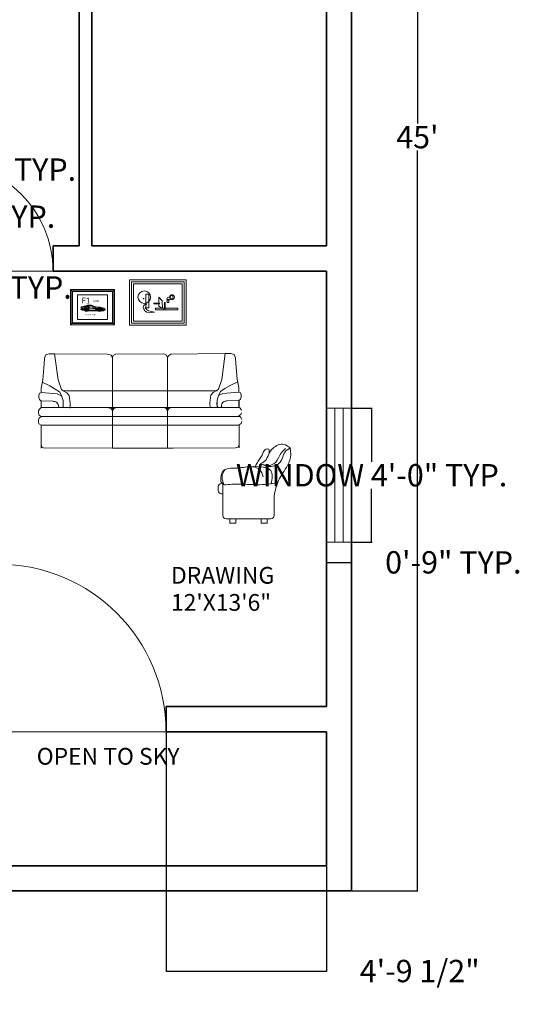
# Model space of a CAD drawing. Units: inches. Extents: x 125 to 976, y 231 to 853.
# Tile 15 of 16: x 736 to 915, y 231 to 584. Entities that reach past the tile are written whole.
import ezdxf

# ---------------------------------------------------------------- set-up
doc = ezdxf.new("R2010")
doc.units = ezdxf.units.IN
doc.header["$MEASUREMENT"] = 0
for name, color, linetype, lineweight in [('A-ANNO-DIMS', 2, 'Continuous', 18), ('A-AREA-IDEN', 7, 'Continuous', 18), ('A-DOOR', 3, 'Continuous', 18), ('A-FURN-ARTW', 9, 'Continuous', 13), ('A-GLAZ', 4, 'Continuous', 18), ('A-WALL', 7, 'Continuous', 35), ('Furniture', 8, 'Continuous', 15)]:
    doc.layers.add(name, color=color, linetype=linetype, lineweight=lineweight)
doc.styles.add('ITALICC', font='italicc', dxfattribs={"height": 240})
doc.styles.get("Standard").update_dxf_attribs({"font": 'italic8.shx'})
doc.dimstyles.get("Standard").update_dxf_attribs({"dimtxt": 8, "dimasz": 0.18, "dimexe": 0.18, "dimexo": 0.0625, "dimgap": 0.09, "dimtad": 0, "dimtih": 1, "dimtoh": 1, "dimdec": 4, "dimzin": 0, "dimdsep": 46, "dimlunit": 3, "dimtxsty": 'Standard', "dimcen": 0.09, "dimclrt": 4, "dimadec": 0, "dimazin": 0, "dimtfac": 1, "dimtdec": 4, "dimtofl": 0, "dimtmove": 0, "dimatfit": 3, "dimfxl": 1, "dimtolj": 1, "dimtzin": 0, "dimarcsym": 0})

# ---------------------------------------------------------------- blocks, each defined once
blk = doc.blocks.new('*D6')
at = {"layer": 'A-ANNO-DIMS', "color": 0, "lineweight": -2, "transparency": 16777216}
for p, q in [((855.26, 812.1), (878.96, 812.1)), ((878.78, 811.92), (878.78, 546.96)), ((878.78, 272.28), (878.78, 537.25)), ((846.26, 272.1), (878.96, 272.1))]:
    blk.add_line(p, q, dxfattribs=at)
at = {"layer": 'A-ANNO-DIMS', "color": 0, "transparency": 16777216}
for points in [[(878.75, 811.92), (878.81, 811.92), (878.78, 812.1)], [(878.75, 272.28), (878.81, 272.28), (878.78, 272.1)]]:
    blk.add_solid(points, dxfattribs=at)
at = {"layer": 'Defpoints', "color": 0, "transparency": 16777216}
for p in [(855.19, 812.1), (846.19, 272.1), (878.78, 272.1)]:
    blk.add_point(p, dxfattribs=at)
at = {"layer": 'A-ANNO-DIMS', "color": 0, "transparency": 16777216, "insert": (878.78, 542.1), "char_height": 8, "attachment_point": 5}
blk.add_mtext("\\A1;45'", dxfattribs=at)
blk = doc.blocks.new('SOFA-3SEAT')
for p, q in [((2, 30.21, -13.5), (2.15, 32.26, -13.5)), ((2.15, 32.26, -13.5), (2.61, 33.47, -13.5)), ((2.61, 33.47, -13.5), (3.76, 33.83, -13.5)), ((3.76, 33.83, -13.5), (5.77, 33.83, -13.5)), ((5.77, 33.83, -13.5), (24.71, 33.77, -13.5)), ((5.77, 33.83, -13.5), (7.07, 24.49, -13.5)), ((24.71, 33.77, -13.5), (26.18, 33.35, -13.5)), ((26.04, 33.37, -13.5), (26.5, 32.59, -13.5)), ((26.43, 32.53, -13.5), (26.87, 33.35, -13.5)), ((26.46, 32.58, -13.5), (26.52, 32.42, -13.5)), ((26.58, 32.81, -13.5), (26.58, 0, -13.5)), ((26.87, 33.35, -13.5), (27.73, 33.77, -13.5)), ((27.73, 33.77, -13.5), (44.96, 33.81, -13.5)), ((45.83, 33.4, -13.5), (44.96, 33.81, -13.5)), ((46.26, 32.57, -13.5), (45.83, 33.4, -13.5)), ((46.23, 32.63, -13.5), (46.18, 32.47, -13.5)), ((46.26, 32.63, -13.5), (46.69, 33.25, -13.5)), ((46.27, 0, -13.5), (46.27, 32.64, -13.5)), ((46.69, 33.25, -13.5), (47.38, 33.77, -13.5)), ((47.38, 33.77, -13.5), (66.92, 33.97, -13.5)), ((63.98, 33.86, -13.5), (63.98, 33.83, -13.5)), ((66.92, 33.97, -13.5), (65.66, 24.62, -13.5)), ((68.93, 33.98, -13.5), (66.92, 33.97, -13.5)), ((70.09, 33.62, -13.5), (68.93, 33.98, -13.5)), ((70.54, 32.42, -13.5), (70.09, 33.62, -13.5)), ((70.7, 30.37, -13.5), (70.54, 32.42, -13.5)), ((1.55, 24.55, -13.5), (2, 30.21, -13.5)), ((71.18, 24.71, -13.5), (70.7, 30.37, -13.5)), ((71.76, 21.75, -13.5), (71.18, 24.71, -13.5)), ((0.99, 21.59, -13.5), (1.55, 24.55, -13.5)), ((0.99, 21.59, -13.5), (0.99, 19.94, -13.5)), ((1.35, 23.64, -13.5), (4.11, 22.38, -13.5)), ((4.11, 22.38, -13.5), (5.97, 21.23, -13.5)), ((5.97, 21.23, -13.5), (7.53, 20.21, -13.5)), ((7.07, 24.49, -13.5), (8.28, 21.05, -13.5)), ((64.47, 21.18, -13.5), (63.92, 20.76, -13.5)), ((65.66, 24.62, -13.5), (64.47, 21.18, -13.5)), ((66.78, 21.37, -13.5), (65.23, 20.34, -13.5)), ((68.63, 22.53, -13.5), (66.78, 21.37, -13.5)), ((71.39, 23.81, -13.5), (68.63, 22.53, -13.5)), ((71.76, 21.75, -13.5), (71.76, 20.1, -13.5)), ((0.14, 18.15, -13.5), (0.18, 18.99, -13.5)), ((0.35, 17.44, -13.5), (0.14, 18.15, -13.5)), ((0.18, 18.99, -13.5), (0.38, 19.7, -13.5)), ((0.38, 19.7, -13.5), (0.98, 19.91, -13.5)), ((0.65, 19.79, -13.5), (0.65, 19.8, -13.5)), ((0.96, 19.94, -13.5), (6.7, 19.5, -13.5)), ((6.7, 19.5, -13.5), (8.26, 18.79, -13.5)), ((7.53, 20.21, -13.5), (8.33, 18.64, -13.5)), ((8.26, 18.79, -13.5), (8.83, 17.11, -13.5)), ((8.28, 21.05, -13.5), (8.83, 20.63, -13.5)), ((8.83, 20.63, -13.5), (63.95, 20.63, -13.5)), ((8.83, 20.63, -13.5), (10.14, 19.91, -13.5)), ((8.86, 20.63, -13.5), (8.86, 20.61, -13.5)), ((10.14, 19.91, -13.5), (10.98, 18.9, -13.5)), ((10.98, 18.9, -13.5), (11.34, 16.01, -13.5)), ((61.78, 19.02, -13.5), (61.43, 16.13, -13.5)), ((62.62, 20.03, -13.5), (61.78, 19.02, -13.5)), ((63.92, 20.76, -13.5), (62.62, 20.03, -13.5)), ((63.89, 20.76, -13.5), (63.89, 20.74, -13.5)), ((64.5, 18.92, -13.5), (63.94, 17.24, -13.5)), ((65.23, 20.34, -13.5), (64.43, 18.77, -13.5)), ((66.05, 19.64, -13.5), (64.5, 18.92, -13.5)), ((71.8, 20.1, -13.5), (66.05, 19.64, -13.5)), ((72.37, 19.87, -13.5), (71.78, 20.07, -13.5)), ((72.11, 19.95, -13.5), (72.11, 19.96, -13.5)), ((72.58, 19.16, -13.5), (72.37, 19.87, -13.5)), ((72.41, 17.61, -13.5), (72.62, 18.32, -13.5)), ((72.62, 18.32, -13.5), (72.58, 19.16, -13.5)), ((0.04, 13.5, -13.5), (0.49, 14.17, -13.5)), ((0.98, 16.94, -13.5), (0.35, 17.44, -13.5)), ((0.49, 14.17, -13.5), (1.01, 14.59, -13.5)), ((0.98, 16.95, -13.5), (5.28, 16.85, -13.5)), ((0.99, 16.95, -13.5), (0.99, 14.57, -13.5)), ((0.99, 14.57, -13.5), (0.99, 16.93, -13.5)), ((0.99, 14.57, -13.5), (71.86, 14.57, -13.5)), ((0.99, 14.57, -13.5), (0.99, 14.57, -13.5)), ((5.51, 16.75, -13.5), (5.27, 16.91, -13.5)), ((7.07, 14.84, -13.5), (7.3, 14.56, -13.5)), ((8.66, 14.72, -13.5), (8.26, 14.56, -13.5)), ((8.83, 14.88, -13.5), (8.66, 14.72, -13.5)), ((8.86, 15.75, -13.5), (8.81, 14.86, -13.5)), ((8.83, 17.11, -13.5), (8.86, 15.72, -13.5)), ((8.89, 14.57, -13.5), (8.89, 14.52, -13.5)), ((11.34, 16.01, -13.5), (11.34, 14.42, -13.5)), ((25.14, 14.53, -13.5), (26.09, 14.22, -13.5)), ((26.09, 14.22, -13.5), (26.52, 13.5, -13.5)), ((26.52, 13.5, -13.5), (27.04, 14.22, -13.5)), ((27.04, 14.22, -13.5), (27.73, 14.53, -13.5)), ((45.74, 14.26, -13.5), (45.05, 14.57, -13.5)), ((45.14, 14.53, -13.5), (46.17, 14.12, -13.5)), ((46.26, 13.54, -13.5), (45.74, 14.26, -13.5)), ((46.17, 14.12, -13.5), (46.26, 13.39, -13.5)), ((46.69, 14.27, -13.5), (46.26, 13.54, -13.5)), ((46.26, 13.39, -13.5), (46.6, 14.12, -13.5)), ((46.6, 14.12, -13.5), (47.29, 14.53, -13.5)), ((47.64, 14.58, -13.5), (46.69, 14.27, -13.5)), ((61.43, 16.13, -13.5), (61.44, 14.54, -13.5)), ((63.88, 14.69, -13.5), (63.88, 14.65, -13.5)), ((63.94, 17.24, -13.5), (63.91, 15.85, -13.5)), ((63.91, 15.87, -13.5), (63.97, 14.99, -13.5)), ((63.95, 15.01, -13.5), (64.12, 14.85, -13.5)), ((63.98, 17.37, -13.5), (63.98, 14.57, -13.5)), ((64.12, 14.85, -13.5), (64.51, 14.69, -13.5)), ((65.71, 14.98, -13.5), (65.48, 14.7, -13.5)), ((67.26, 16.9, -13.5), (67.49, 17.06, -13.5)), ((71.79, 17.11, -13.5), (67.48, 17, -13.5)), ((72.29, 14.34, -13.5), (71.76, 14.75, -13.5)), ((71.78, 17.11, -13.5), (71.79, 14.73, -13.5)), ((71.79, 14.73, -13.5), (71.78, 17.09, -13.5)), ((71.79, 17.1, -13.5), (72.41, 17.61, -13.5)), ((71.79, 14.73, -13.5), (71.79, 14.74, -13.5)), ((71.86, 17.15, -13.5), (71.86, 14.57, -13.5)), ((72.75, 13.67, -13.5), (72.29, 14.34, -13.5)), ((0.31, 10.84, -13.5), (0, 10.18, -13.5)), ((0.04, 12.58, -13.5), (0.04, 13.5, -13.5)), ((0.31, 11.91, -13.5), (0.04, 12.58, -13.5)), ((0.98, 11.41, -13.5), (0.31, 11.91, -13.5)), ((0.98, 11.45, -13.5), (0.31, 10.84, -13.5)), ((71.86, 11.42, -13.5), (0.99, 11.42, -13.5)), ((71.8, 11.42, -13.5), (71.8, 11.58, -13.5)), ((71.81, 11.57, -13.5), (72.48, 12.08, -13.5)), ((71.82, 11.61, -13.5), (72.49, 11, -13.5)), ((71.86, 11.6, -13.5), (71.86, 11.42, -13.5)), ((71.86, 11.6, -13.5), (71.86, 11.42, -13.5)), ((72.48, 12.08, -13.5), (72.75, 12.75, -13.5)), ((72.49, 11, -13.5), (72.8, 10.35, -13.5)), ((0, 10.18, -13.5), (0, 9.47, -13.5)), ((0, 9.47, -13.5), (0.19, 8.77, -13.5)), ((0.19, 8.77, -13.5), (0.98, 8.25, -13.5)), ((0.99, 8.27, -13.5), (71.86, 8.27, -13.5)), ((0.99, 0, -13.5), (0.99, 8.27, -13.5)), ((0.99, 8.27, -13.5), (0.99, 1.21, -13.5)), ((0.99, 8.27, -13.5), (0.99, 0, -13.5)), ((71.82, 8.43, -13.5), (71.81, 8.27, -13.5)), ((71.86, 0.16, -13.5), (71.82, 8.43, -13.5)), ((71.82, 8.43, -13.5), (71.85, 1.37, -13.5)), ((71.86, 0.16, -13.5), (71.82, 8.27, -13.5)), ((72.61, 8.93, -13.5), (71.83, 8.41, -13.5)), ((71.86, 8.43, -13.5), (71.86, 8.27, -13.5)), ((72.81, 9.64, -13.5), (72.61, 8.93, -13.5)), ((0.99, 1.21, -13.5), (1.35, 0.26, -13.5)), ((1.35, 0.26, -13.5), (2.3, 0, -13.5)), ((2.3, 0, -13.5), (70.55, 0.16, -13.5)), ((71.49, 0.42, -13.5), (70.55, 0.16, -13.5)), ((71.85, 1.37, -13.5), (71.49, 0.42, -13.5)), ((26.58, 0, -13.5), (46.27, 0, -13.5)), ((28.55, 0, -13.5), (48.23, 0, -13.5))]:
    blk.add_line(p, q)
for centre, start, end in [((5.4, 14.95, -13.5), 347.9294, 88.2763), ((67.38, 15.1, -13.5), 91.9867, 192.3335)]:
    blk.add_arc(centre, 1.85, start, end)
blk = doc.blocks.new('ART-FRAMED-ABSTRACT')
for p, q in [((0, 16.18), (20.24, 16.18)), ((0, 0), (0, 16.18)), ((0.71, 15.47), (19.53, 15.47)), ((0.71, 0.71), (0.71, 15.47)), ((0.71, 15.47), (19.53, 15.47)), ((0.71, 0.71), (0.71, 15.47)), ((1.42, 14.76), (18.82, 14.76)), ((1.42, 1.42), (1.42, 14.76)), ((18.82, 14.76), (18.82, 1.42)), ((19.53, 15.47), (19.53, 0.71)), ((19.53, 15.47), (19.53, 0.71)), ((20.24, 16.18), (20.24, 0)), ((5.79, 11.06), (6.88, 11.06)), ((5.79, 6.17), (5.79, 11.06)), ((6.88, 11.06), (6.88, 6.17)), ((6.88, 10.8), (6.95, 10.83)), ((6.88, 10.62), (6.95, 10.83)), ((3.12, 9.36), (3.17, 9.38)), ((3.14, 9.3), (3.17, 9.37)), ((4.91, 9.37), (5.13, 9.63)), ((4.91, 9.37), (5.18, 9.35)), ((5.18, 9.34), (5.13, 9.63)), ((5.66, 7.36), (5.76, 7.29)), ((5.76, 7.29), (5.79, 7.36)), ((5.79, 7.54), (5.85, 7.56)), ((5.81, 7.44), (5.85, 7.56)), ((8.71, 7.89), (10.73, 7.89)), ((8.71, 7.59), (8.71, 7.89)), ((10.73, 7.59), (8.71, 7.59)), ((10.55, 10.02), (11.64, 8.68)), ((10.55, 6.72), (10.55, 10.02)), ((10.73, 7.89), (10.73, 7.59)), ((11.64, 8.68), (11.75, 5.9)), ((12.76, 8.08), (12.51, 8.08)), ((12.51, 8.08), (12.51, 5.81)), ((12.76, 5.81), (12.76, 8.08)), ((13.43, 8.14), (13.43, 9.18)), ((13.43, 9.18), (14.11, 9.18)), ((14.11, 8.14), (13.43, 8.14)), ((14.11, 9.18), (14.11, 8.14)), ((5.53, 5.99), (5.8, 5.96)), ((5.54, 5.99), (5.75, 6.25)), ((5.81, 5.96), (5.75, 6.24)), ((6.88, 6.17), (5.79, 6.17)), ((17.28, 6.04), (9.28, 6.04)), ((9.28, 6.04), (9.28, 5.49)), ((9.28, 5.49), (17.28, 5.49)), ((11.75, 5.9), (10.55, 6.72)), ((12.04, 5.49), (12.21, 5.68)), ((12.24, 5.49), (12.21, 5.68)), ((12.51, 5.81), (12.76, 5.81)), ((17.28, 5.49), (17.28, 6.04)), ((20.24, 0), (0, 0)), ((19.53, 0.71), (0.71, 0.71)), ((19.53, 0.71), (0.71, 0.71)), ((18.82, 1.42), (1.42, 1.42))]:
    blk.add_line(p, q)
for centre, radius in [((5.29, 9.99), 2.26), ((15.21, 9.98), 0.893), ((13.98, 9.43), 0.565), ((15.09, 9.98), 0.578)]:
    blk.add_circle(centre, radius)
for points, knots in [([(6.1, 7.58), (5.6, 7.34), (4.53, 6.82), (5.68, 4.07), (7.64, 4.38), (8.96, 4.59)], [0, 0, 0, 0, 1.44737, 3.141992, 6.657621, 6.657621, 6.657621, 6.657621]), ([(6.1, 7.58), (5.92, 7.07), (5.29, 5.32), (7.43, 4.89), (8.96, 4.59)], [0, 0, 0, 0, 1.438871, 4.981716, 4.981716, 4.981716, 4.981716])]:
    blk.add_open_spline(points, degree=3, knots=knots)
blk = doc.blocks.new('WINDOW-48IN')
for p, q in [((0, 0), (0, 48)), ((0, 48), (9, 48)), ((3, 0), (3, 48)), ((6, 0), (6, 48)), ((9, 48), (9, 0)), ((9, 0), (0, 0))]:
    blk.add_line(p, q)
blk = doc.blocks.new('DOOR-39IN-RH')
for p, q in [((0, 39), (0, 0)), ((2, 38.95), (2, 0)), ((0, 0), (39, 0))]:
    blk.add_line(p, q)
blk.add_arc((0, 0), 39, 0, 90)
blk = doc.blocks.new('DOOR-60IN')
for p, q in [((0, 0), (0, 60)), ((2, 0), (2, 59.97)), ((60, 0), (0, 0))]:
    blk.add_line(p, q)
blk.add_arc((0, 0), 60, 0, 90)
blk = doc.blocks.new('*D24')
at = {"layer": 'A-ANNO-DIMS', "color": 0, "lineweight": -2, "transparency": 16777216}
for p, q in [((855.26, 444.98), (862.57, 444.98)), ((862.39, 444.8), (862.39, 425.84)), ((862.39, 397.16), (862.39, 416.13)), ((855.26, 396.98), (862.57, 396.98))]:
    blk.add_line(p, q, dxfattribs=at)
at = {"layer": 'A-ANNO-DIMS', "color": 0, "transparency": 16777216}
for points in [[(862.36, 444.8), (862.42, 444.8), (862.39, 444.98)], [(862.36, 397.16), (862.42, 397.16), (862.39, 396.98)]]:
    blk.add_solid(points, dxfattribs=at)
at = {"layer": 'Defpoints', "color": 0, "transparency": 16777216}
for p in [(855.19, 444.98), (862.39, 444.98), (855.19, 396.98)]:
    blk.add_point(p, dxfattribs=at)
at = {"layer": 'A-ANNO-DIMS', "color": 4, "transparency": 16777216, "insert": (862.39, 420.98), "char_height": 8, "attachment_point": 5}
blk.add_mtext('\\A1;WINDOW 4\'-0" TYP.', dxfattribs=at)
blk = doc.blocks.new('*D25')
at = {"layer": 'A-ANNO-DIMS', "color": 0, "lineweight": -2, "transparency": 16777216}
for p, q in [((846.19, 396.92), (846.19, 389.6)), ((855.19, 396.92), (855.19, 389.6)), ((846.37, 389.78), (855.01, 389.78)), ((855.19, 389.78), (855.37, 389.78))]:
    blk.add_line(p, q, dxfattribs=at)
at = {"layer": 'A-ANNO-DIMS', "color": 0, "transparency": 16777216}
for points in [[(846.37, 389.81), (846.37, 389.75), (846.19, 389.78)], [(855.01, 389.81), (855.01, 389.75), (855.19, 389.78)]]:
    blk.add_solid(points, dxfattribs=at)
at = {"layer": 'Defpoints', "color": 0, "transparency": 16777216}
for p in [(846.19, 396.98), (855.19, 396.98), (855.19, 389.78)]:
    blk.add_point(p, dxfattribs=at)
at = {"layer": 'A-ANNO-DIMS', "color": 4, "transparency": 16777216, "insert": (891.65, 389.78), "char_height": 8, "attachment_point": 5}
blk.add_mtext('\\A1;0\'-9" TYP.', dxfattribs=at)
blk = doc.blocks.new('*D38')
at = {"layer": 'A-ANNO-DIMS', "color": 0, "lineweight": -2, "transparency": 16777216}
for p, q in [((694.22, 533.1), (700.18, 533.1)), ((700, 532.92), (700, 518.46)), ((700, 494.28), (700, 508.75)), ((694.22, 494.1), (700.18, 494.1))]:
    blk.add_line(p, q, dxfattribs=at)
at = {"layer": 'A-ANNO-DIMS', "color": 0, "transparency": 16777216}
for points in [[(699.97, 532.92), (700.03, 532.92), (700, 533.1)], [(699.97, 494.28), (700.03, 494.28), (700, 494.1)]]:
    blk.add_solid(points, dxfattribs=at)
at = {"layer": 'Defpoints', "color": 0, "transparency": 16777216}
for p in [(694.15, 533.1), (700, 533.1), (694.15, 494.1)]:
    blk.add_point(p, dxfattribs=at)
at = {"layer": 'A-ANNO-DIMS', "color": 4, "transparency": 16777216, "insert": (700, 513.6), "char_height": 8, "attachment_point": 5}
blk.add_mtext('\\A1;LH DOOR 3\'-3" TYP.', dxfattribs=at)
blk = doc.blocks.new('*D39')
at = {"layer": 'A-ANNO-DIMS', "color": 0, "lineweight": -2, "transparency": 16777216}
for p, q in [((655.15, 494.04), (655.15, 488.07)), ((694.15, 494.04), (694.15, 488.07)), ((655.33, 488.25), (693.97, 488.25)), ((694.15, 488.25), (694.33, 488.25))]:
    blk.add_line(p, q, dxfattribs=at)
at = {"layer": 'A-ANNO-DIMS', "color": 0, "transparency": 16777216}
for points in [[(655.33, 488.28), (655.33, 488.22), (655.15, 488.25)], [(693.97, 488.28), (693.97, 488.22), (694.15, 488.25)]]:
    blk.add_solid(points, dxfattribs=at)
at = {"layer": 'Defpoints', "color": 0, "transparency": 16777216}
for p in [(655.15, 494.1), (694.15, 494.1), (694.15, 488.25)]:
    blk.add_point(p, dxfattribs=at)
at = {"layer": 'A-ANNO-DIMS', "color": 4, "transparency": 16777216, "insert": (730.61, 488.25), "char_height": 8, "attachment_point": 5}
blk.add_mtext('\\A1;3\'-3" TYP.', dxfattribs=at)
blk = doc.blocks.new('*D48')
at = {"layer": 'A-ANNO-DIMS', "color": 0, "lineweight": -2, "transparency": 16777216}
for p, q in [((609.57, 526.38), (609.57, 530.63)), ((609.75, 530.45), (636.95, 530.45)), ((637.13, 526.38), (637.13, 530.63)), ((637.13, 530.45), (637.31, 530.45))]:
    blk.add_line(p, q, dxfattribs=at)
at = {"layer": 'A-ANNO-DIMS', "color": 0, "transparency": 16777216}
for points in [[(609.75, 530.48), (609.75, 530.42), (609.57, 530.45)], [(636.95, 530.48), (636.95, 530.42), (637.13, 530.45)]]:
    blk.add_solid(points, dxfattribs=at)
at = {"layer": 'Defpoints', "color": 0, "transparency": 16777216}
for p in [(637.13, 530.45), (609.57, 526.32), (637.13, 526.32)]:
    blk.add_point(p, dxfattribs=at)
at = {"layer": 'A-ANNO-DIMS', "color": 4, "transparency": 16777216, "insert": (709.21, 530.45), "char_height": 8, "attachment_point": 5}
blk.add_mtext('\\A1;SINK 2\'-3 1/2" TYP.', dxfattribs=at)
blk = doc.blocks.new('*D61')
at = {"layer": 'A-ANNO-DIMS', "color": 0, "lineweight": -2, "transparency": 16777216}
for p, q in [((788.78, 329.04), (788.78, 243.22)), ((846.19, 329.04), (846.19, 243.22)), ((788.96, 243.4), (846.01, 243.4)), ((846.19, 243.4), (846.37, 243.4))]:
    blk.add_line(p, q, dxfattribs=at)
at = {"layer": 'A-ANNO-DIMS', "color": 0, "transparency": 16777216}
for points in [[(788.96, 243.43), (788.96, 243.37), (788.78, 243.4)], [(846.01, 243.43), (846.01, 243.37), (846.19, 243.4)]]:
    blk.add_solid(points, dxfattribs=at)
at = {"layer": 'Defpoints', "color": 0, "transparency": 16777216}
for p in [(788.78, 329.1), (846.19, 329.1), (846.19, 243.4)]:
    blk.add_point(p, dxfattribs=at)
at = {"layer": 'A-ANNO-DIMS', "color": 4, "transparency": 16777216, "insert": (879.61, 243.4), "char_height": 8, "attachment_point": 5}
blk.add_mtext('\\A1;4\'-9 1/2"', dxfattribs=at)

msp = doc.modelspace()

# ---------------------------------------------------------------- linework, layer by layer
at = {"layer": 'A-FURN-ARTW'}
for p, q in [((754.60231, 487.494), (770.35031, 487.494)), ((754.60231, 487.494), (754.60231, 474.8956)), ((755.29522, 486.80109), (754.60231, 487.494)), ((755.07475, 487.02156), (769.87787, 487.02156)), ((755.07475, 487.02156), (755.07475, 475.36804)), ((755.23223, 486.86408), (769.72039, 486.86408)), ((755.23223, 486.86408), (755.23223, 475.52552)), ((755.29522, 486.80109), (769.6574, 486.80109)), ((755.29522, 486.80109), (755.29522, 475.58851)), ((769.6574, 486.80109), (770.35031, 487.494)), ((769.6574, 486.80109), (769.6574, 475.58851)), ((769.72039, 486.86408), (769.72039, 475.52552)), ((769.87787, 487.02156), (769.87787, 475.36804)), ((770.35031, 487.494), (770.35031, 474.8956)), ((757.12199, 485.60424), (767.83063, 485.60424)), ((757.12199, 485.60424), (757.12199, 476.78536)), ((767.83063, 485.60424), (767.83063, 476.78536)), ((758.28026, 480.5186), (758.34094, 480.76133)), ((758.31237, 480.5105), (758.28291, 480.5105)), ((758.3117, 480.42103), (758.28293, 480.4868)), ((758.33795, 480.50224), (758.31237, 480.5105)), ((758.33128, 480.50425), (759.47693, 480.30077)), ((758.33229, 480.52296), (758.39189, 480.76133)), ((758.38079, 480.38642), (758.33496, 480.49117)), ((758.36266, 481.31769), (758.41208, 480.89761)), ((758.38737, 480.83583), (758.41208, 480.89761)), ((758.39972, 480.81112), (758.38737, 480.83583)), ((758.38737, 480.78641), (758.39972, 480.81112)), ((758.38889, 480.83583), (759.73849, 480.83583)), ((758.38889, 480.79877), (759.73214, 480.79877)), ((758.41544, 481.29201), (758.46263, 480.89091)), ((758.4406, 480.83583), (758.46263, 480.89091)), ((758.45824, 480.30563), (759.47462, 480.12512)), ((758.71184, 480.14222), (758.57964, 480.20951)), ((758.7086, 480.83583), (758.65918, 481.30533)), ((758.75802, 480.74935), (758.75802, 480.65051)), ((758.75802, 480.74935), (759.09161, 480.74935)), ((758.75802, 480.65051), (759.09161, 480.65051)), ((758.77379, 481.30451), (759.74709, 481.35476)), ((758.83434, 480.20886), (758.8198, 480.24279)), ((758.9079, 480.15048), (759.62949, 480.02232)), ((759.09161, 480.74935), (759.09161, 480.65051)), ((759.15339, 481.37946), (759.74644, 481.37946)), ((759.47462, 480.24279), (759.47462, 480.12512)), ((760.68637, 481.36279), (760.62387, 481.83335)), ((760.71087, 481.36605), (760.64837, 481.8366)), ((760.66826, 480.83615), (764.36543, 480.6804)), ((760.67502, 480.79877), (764.37001, 480.6431)), ((760.75956, 479.88449), (761.03138, 479.88449)), ((761.0808, 479.93391), (760.77192, 479.9092)), ((762.28859, 481.82292), (760.92169, 481.79935)), ((761.05609, 481.3424), (760.92169, 481.79935)), ((760.95361, 479.97939), (760.93253, 480.24279)), ((762.00687, 481.79335), (760.95455, 481.7752)), ((761.07979, 481.34937), (760.95455, 481.7752)), ((760.95725, 480.13159), (764.24854, 480.13159)), ((760.95725, 479.98333), (764.21901, 479.98333)), ((761.00287, 479.93391), (764.21901, 479.93391)), ((761.03138, 479.88449), (761.09315, 479.9092)), ((761.72327, 481.26827), (761.05609, 481.3424)), ((761.0808, 481.13236), (761.37732, 481.13236)), ((761.0808, 481.04587), (761.0808, 481.13236)), ((761.37732, 481.08294), (761.0808, 481.08294)), ((761.37732, 481.04587), (761.0808, 481.04587)), ((761.09315, 479.9092), (761.34026, 479.9092)), ((761.34026, 479.9092), (761.35261, 479.87213)), ((761.35261, 479.87213), (761.82211, 479.87213)), ((761.37732, 481.13236), (761.37732, 481.04587)), ((761.82211, 479.87213), (761.92095, 479.88449)), ((761.92095, 479.88449), (762.01979, 479.89684)), ((761.96424, 481.81733), (763.01468, 481.22646)), ((762.01314, 481.81817), (763.06137, 481.22854)), ((762.01979, 479.89684), (762.09392, 479.89684)), ((762.09392, 479.89684), (762.11863, 479.87213)), ((762.11095, 481.81986), (763.15355, 481.23339)), ((762.11863, 479.87213), (762.20512, 479.87213)), ((762.20512, 479.87213), (762.2916, 479.88449)), ((762.28859, 481.82292), (763.50241, 481.26065)), ((762.2916, 479.88449), (762.45222, 479.88449)), ((762.45222, 479.88449), (762.46458, 479.87213)), ((762.46458, 479.87213), (762.56342, 479.87213)), ((762.5669, 481.39311), (762.52131, 481.22594)), ((762.56342, 479.87213), (762.60048, 479.88449)), ((762.63842, 481.37361), (762.59625, 481.21898)), ((762.60048, 479.88449), (763.28002, 479.88449)), ((762.66226, 481.36711), (762.62519, 481.2312)), ((762.62519, 481.2312), (762.6499, 481.20649)), ((762.62519, 481.2312), (762.94643, 481.2312)), ((762.6499, 481.20649), (762.92172, 481.21885)), ((762.67461, 481.39182), (762.66226, 481.36711)), ((762.95878, 481.2312), (762.66226, 481.35475)), ((762.95878, 481.2312), (762.67461, 481.39182)), ((762.71168, 481.18178), (762.71168, 481.21885)), ((762.85994, 481.18178), (762.71168, 481.18178)), ((762.85994, 481.21885), (762.85994, 481.18178)), ((764.68851, 481.19413), (762.85994, 481.19413)), ((762.92172, 481.21885), (762.95878, 481.2312)), ((763.28002, 479.88449), (763.30473, 479.87213)), ((763.30473, 479.87213), (763.40357, 479.87213)), ((763.40357, 479.87213), (763.41593, 479.88449)), ((763.41593, 479.88449), (763.78658, 479.89684)), ((763.57173, 481.26606), (764.47103, 481.19413)), ((763.73716, 480.20572), (763.62596, 480.20572)), ((763.76187, 480.58873), (763.63832, 480.58873)), ((763.70377, 481.3041), (763.6908, 481.25518)), ((763.73558, 481.30145), (763.70377, 481.3041)), ((763.74492, 481.28939), (763.73558, 481.30145)), ((763.76187, 480.58873), (763.73716, 480.20572)), ((763.74492, 481.28939), (764.68851, 481.19413)), ((763.78658, 479.89684), (764.1943, 479.89684)), ((763.98426, 480.20572), (763.87307, 480.20572)), ((764.00897, 480.57638), (763.88542, 480.57638)), ((764.00897, 480.57638), (763.98426, 480.20572)), ((764.1943, 479.89684), (764.26843, 479.89684)), ((764.24854, 480.13159), (764.21901, 479.98333)), ((764.21901, 479.98333), (764.21901, 479.93391)), ((764.26843, 479.89684), (764.29314, 479.92155)), ((764.29314, 479.92155), (764.36727, 479.9092)), ((764.36727, 479.9092), (764.41669, 479.9092)), ((764.41669, 479.9092), (764.43723, 479.91946)), ((765.57808, 479.92155), (765.52906, 479.91338)), ((765.65221, 479.94626), (765.57808, 479.92155)), ((765.75105, 479.9092), (765.65221, 479.94626)), ((765.70762, 480.58675), (766.67803, 480.54587)), ((765.71532, 480.62353), (766.66898, 480.58335)), ((765.81283, 479.9092), (765.75105, 479.9092)), ((765.81283, 480.03275), (765.79911, 480.26415)), ((765.81283, 480.03275), (765.81283, 479.85978)), ((765.87531, 480.53022), (766.20417, 480.51637)), ((765.87531, 480.53022), (765.9003, 480.43024)), ((765.9003, 480.43024), (766.24186, 480.41585)), ((766.20417, 480.51637), (766.24186, 480.41585)), ((766.3018, 479.89084), (766.40588, 479.98333)), ((766.40588, 479.98333), (766.61592, 480.05746)), ((766.61592, 480.05746), (766.66534, 480.10688)), ((766.66898, 480.58335), (766.75364, 480.2326)), ((766.67803, 480.54587), (766.88975, 480.56691)), ((766.70701, 480.586), (766.84673, 480.59988)), ((766.7307, 480.48561), (766.77734, 480.2924)), ((766.75228, 480.516), (766.89341, 480.53002)), ((766.76418, 480.16866), (766.80124, 480.19337)), ((766.76677, 480.33617), (766.92479, 480.30456)), ((766.87537, 480.30456), (766.77678, 480.2947)), ((766.78365, 480.26623), (766.80124, 480.19337)), ((766.7897, 480.19625), (766.90008, 480.16866)), ((766.94951, 480.30456), (766.87537, 480.30456)), ((766.89341, 480.53002), (766.94951, 480.30456)), ((766.91471, 480.54296), (766.98479, 480.27431)), ((757.12199, 476.78536), (767.83063, 476.78536)), ((755.29522, 475.58851), (754.60231, 474.8956)), ((754.60231, 474.8956), (770.35031, 474.8956)), ((755.07475, 475.36804), (769.87787, 475.36804)), ((755.23223, 475.52552), (769.72039, 475.52552)), ((755.29522, 475.58851), (769.6574, 475.58851)), ((769.6574, 475.58851), (770.35031, 474.8956))]:
    msp.add_line(p, q, dxfattribs=at)
for centre, radius in [((760.22829, 480.25514), 0.64247), ((760.22829, 480.25514), 0.49421), ((760.22829, 480.25514), 0.44479), ((760.22829, 480.25514), 0.2471), ((760.22829, 480.25514), 0.19768), ((760.08003, 480.25514), 0.02471), ((760.22829, 480.25514), 0.07413), ((760.18247, 480.39615), 0.02471), ((760.18247, 480.11414), 0.02471), ((760.34824, 480.34229), 0.02471), ((760.34824, 480.168), 0.02471), ((764.98503, 480.25514), 0.64247), ((764.98503, 480.25514), 0.49421), ((764.98503, 480.25514), 0.44479), ((764.98503, 480.25514), 0.2471), ((764.98503, 480.25514), 0.19768), ((764.83677, 480.25514), 0.02471), ((764.98503, 480.25514), 0.07413), ((764.93922, 480.39615), 0.02471), ((764.93922, 480.11414), 0.02471), ((765.10498, 480.34229), 0.02471), ((765.10498, 480.168), 0.02471)]:
    msp.add_circle(centre, radius, dxfattribs=at)
for centre, radius, start, end in [((758.32821, 480.50661), 0.04942, 165.9637565, 203.6293777), ((758.49281, 480.50027), 0.19768, 203.6293777, 259.9289375), ((758.38024, 480.51098), 0.04942, 165.9637565, 203.6293777), ((758.38889, 480.74935), 0.04942, 90, 165.9637565), ((758.45963, 485.16796), 3.85149, 268.5572, 280.3771181), ((758.37356, 481.26891), 0.04783, 28.8809621, 100.3164566), ((757.77157, 481.03149), 0.64307, 353.8619855, 19.3390879), ((758.51662, 480.44585), 0.14826, 203.6293777, 259.9289375), ((758.43983, 480.74935), 0.04942, 90, 165.9637565), ((757.78767, 481.03149), 0.64307, 353.8619855, 19.3390879), ((758.88575, 481.1779), 0.4815, 179.5142446, 197.7013491), ((758.45963, 485.16796), 3.8762, 269.3467381, 274.6487218), ((758.85814, 480.10092), 0.29891, 143.8021327, 158.6989451), ((758.82923, 480.12635), 0.11845, 100.5968558, 172.3030214), ((758.92519, 480.2478), 0.09884, 203.1985905, 259.9289375), ((763.44988, 470.16664), 12.00779, 103.37068, 110.9656649), ((760.20358, 480.24279), 0.72896, 0, 180), ((760.20358, 480.48989), 0.6054, 34.8499046, 145.1500954), ((760.20358, 480.24279), 0.75367, 51.9345418, 128.1046218), ((760.0615, 469.35582), 12.02777, 85.2567236, 91.5009845), ((760.0615, 469.35582), 12.00306, 84.4178875, 91.5009845), ((760.22829, 480.25514), 0.42008, 155.4545455, 178.5415782), ((760.22829, 480.25514), 0.42008, 188.1818182, 211.268851), ((760.22829, 480.25514), 0.39537, 159.1289708, 182.4346937), ((760.22829, 480.25514), 0.39537, 191.8562435, 215.1619665), ((760.22829, 480.25514), 0.37066, 161.8383609, 185.4083365), ((760.22829, 480.25514), 0.37066, 194.5656336, 218.1356092), ((760.22829, 480.25514), 0.42008, 122.7272727, 145.8143055), ((760.22829, 480.25514), 0.39537, 126.4016981, 149.707421), ((760.22829, 480.25514), 0.37066, 129.1110882, 152.6810638), ((760.22829, 480.25514), 0.42008, 220.9090909, 243.9961237), ((760.22829, 480.25514), 0.39537, 224.5835162, 247.8892392), ((760.22829, 480.25514), 0.37066, 227.2929063, 250.862882), ((760.22829, 480.25514), 0.37066, 96.3838154, 119.953791), ((760.22829, 480.25514), 0.39537, 93.6744253, 116.9801483), ((760.22829, 480.25514), 0.42008, 90, 113.0870328), ((760.22829, 480.25514), 0.42008, 253.6363636, 276.7233964), ((760.22829, 480.25514), 0.39537, 257.310789, 280.6165119), ((760.22829, 480.25514), 0.37066, 260.0201791, 283.5901547), ((760.22829, 480.25514), 0.37066, 63.6565427, 87.2265183), ((760.22829, 480.25514), 0.39537, 60.9471526, 84.2528755), ((760.22829, 480.25514), 0.42008, 57.2727273, 80.35976), ((760.22829, 480.25514), 0.42008, 286.3636364, 309.4506691), ((760.22829, 480.25514), 0.39537, 290.0380617, 313.3437846), ((760.22829, 480.25514), 0.37066, 292.7474518, 316.3174274), ((760.22829, 480.25514), 0.37066, 30.92927, 54.4992456), ((760.22829, 480.25514), 0.39537, 28.2198799, 51.5256028), ((760.22829, 480.25514), 0.42008, 24.5454545, 47.6324873), ((760.22829, 480.25514), 0.37066, 325.4747245, 349.0447001), ((760.22829, 480.25514), 0.39537, 322.7653344, 346.0710574), ((760.22829, 480.25514), 0.42008, 319.0909091, 342.1779419), ((760.22829, 480.25514), 0.37066, 358.2019972, 21.7719729), ((760.22829, 480.25514), 0.39537, 355.4926072, 18.7983301), ((760.22829, 480.25514), 0.42008, 351.8181818, 14.9052146), ((761.53098, 474.84465), 7.05665, 86.2290638, 96.9829422), ((761.00265, 481.82129), 0.08388, 138.8611482, 195.1600224), ((761.00287, 479.98333), 0.04942, 184.5739213, 270), ((762.94643, 481.03352), 1.9398, 170.837653, 207.7075506), ((762.6499, 489.92461), 8.7058, 263.8899106, 269.9188598), ((762.0198, 481.28686), 0.59968, 63.3696371, 92.3620858), ((762.60243, 481.3825), 0.03708, 346.1228997, 163.3668629), ((762.6499, 489.92461), 8.7058, 271.8811817, 275.9581755), ((762.79392, 480.61075), 0.77541, 321.8343196, 48.7947718), ((763.56385, 481.16753), 0.09884, 85.4273675, 95.9581755), ((763.65376, 480.38796), 0.20136, 58.1724219, 94.3987054), ((763.90087, 480.3756), 0.20136, 58.1724219, 94.3987054), ((765.0221, 480.21808), 0.77838, 3.3931426, 186.3793702), ((765.0221, 480.21808), 0.80309, 30.3224734, 144.8528028), ((765.02863, 480.37637), 0.72896, 20.2032747, 155.1164342), ((764.98503, 480.25514), 0.42008, 155.4545455, 178.5415782), ((764.98503, 480.25514), 0.42008, 188.1818182, 211.268851), ((764.98503, 480.25514), 0.39537, 159.1289708, 182.4346937), ((764.98503, 480.25514), 0.39537, 191.8562435, 215.1619665), ((764.98503, 480.25514), 0.37066, 161.8383609, 185.4083365), ((764.98503, 480.25514), 0.37066, 194.5656336, 218.1356092), ((764.98503, 480.25514), 0.42008, 122.7272727, 145.8143055), ((764.98503, 480.25514), 0.39537, 126.4016981, 149.707421), ((764.98503, 480.25514), 0.37066, 129.1110882, 152.6810638), ((764.98503, 480.25514), 0.42008, 220.9090909, 243.9961237), ((764.81206, 479.52825), 1.67046, 77.1800811, 94.2416123), ((764.98503, 480.25514), 0.39537, 224.5835162, 247.8892392), ((764.98503, 480.25514), 0.37066, 227.2929063, 250.862882), ((764.98503, 480.25514), 0.37066, 96.3838154, 119.953791), ((764.98503, 480.25514), 0.39537, 93.6744253, 116.9801483), ((764.98503, 480.25514), 0.42008, 90, 113.0870328), ((764.98503, 480.25514), 0.42008, 253.6363636, 276.7233964), ((764.98503, 480.25514), 0.39537, 257.310789, 280.6165119), ((764.98503, 480.25514), 0.37066, 260.0201791, 283.5901547), ((764.98503, 480.25514), 0.37066, 63.6565427, 87.2265183), ((764.98503, 480.25514), 0.39537, 60.9471526, 84.2528755), ((764.98503, 480.25514), 0.42008, 57.2727273, 80.35976), ((764.98503, 480.25514), 0.42008, 286.3636364, 309.4506691), ((764.98503, 480.25514), 0.39537, 290.0380617, 313.3437846), ((764.98503, 480.25514), 0.37066, 292.7474518, 316.3174274), ((763.39448, 472.85829), 8.48926, 65.911013, 77.8397357), ((764.98503, 480.25514), 0.37066, 30.92927, 54.4992456), ((764.98503, 480.25514), 0.39537, 28.2198799, 51.5256028), ((764.98503, 480.25514), 0.42008, 24.5454545, 47.6324873), ((764.98503, 480.25514), 0.37066, 325.4747245, 349.0447001), ((764.98503, 480.25514), 0.39537, 322.7653344, 346.0710574), ((764.98503, 480.25514), 0.42008, 319.0909091, 342.1779419), ((764.98503, 480.25514), 0.37066, 358.2019972, 21.7719729), ((764.98503, 480.25514), 0.39537, 355.4926072, 18.7983301), ((764.98503, 480.25514), 0.42008, 351.8181818, 14.9052146), ((766.15211, 482.06857), 2.0639, 260.5382306, 282.9865514), ((766.2027, 481.56844), 1.75258, 257.1468232, 273.2327012), ((765.99048, 486.03381), 5.91596, 268.7579851, 277.5147317), ((766.30465, 482.68537), 2.60399, 260.2183204, 283.4925926), ((765.06329, 478.34265), 2.75663, 54.3745406, 70.6910807), ((766.58522, 479.93178), 0.35484, 155.0076792, 167.8492948), ((766.58522, 479.93178), 0.30542, 150.5021079, 165.3036108), ((766.58514, 479.85366), 0.28577, 172.5250342, 187.0372829), ((766.59584, 480.60611), 0.14161, 112.4396146, 187.0475111), ((766.75472, 480.49141), 0.02471, 95.6743266, 193.5704344), ((766.80168, 480.2442), 0.04942, 193.5704344, 255.9637565), ((766.81907, 480.51801), 0.09884, 14.620874, 65.911013), ((766.82286, 480.27367), 0.13035, 306.326826, 13.706961), ((766.88915, 480.24936), 0.09884, 283.4925926, 14.620874)]:
    msp.add_arc(centre, radius, start, end, dxfattribs=at)
at = {"layer": 'A-WALL'}
for p, q in [((757.69287, 503.10475), (757.69287, 614.10475)), ((762.19287, 503.10475), (762.19287, 614.10475)), ((846.19287, 614.10475), (846.19287, 503.10475)), ((757.69287, 503.10475), (748.30979, 503.10475)), ((748.30979, 494.10475), (748.30979, 503.10475)), ((846.19287, 503.10475), (762.19287, 503.10475)), ((846.19287, 494.10475), (748.30979, 494.10475)), ((846.19287, 494.10475), (846.19287, 338.10475)), ((846.19287, 338.10475), (788.78314, 338.10475)), ((788.78314, 338.10475), (788.78314, 329.10475)), ((846.19287, 329.10475), (788.78314, 329.10475)), ((846.19287, 329.10475), (846.19287, 281.10475)), ((846.19287, 281.10475), (576.19287, 281.10475))]:
    msp.add_line(p, q, dxfattribs=at)
msp.add_lwpolyline([(567.19287, 812.10475), (855.19287, 812.10475), (855.19287, 272.10475), (567.19287, 272.10475)], close=True, dxfattribs=at)
at = {"layer": 'Furniture'}
for p, q in [((807.49864, 416.89065), (807.49864, 415.48008)), ((808.65971, 418.05172), (808.89559, 418.05172)), ((808.65971, 414.31901), (809.11948, 414.31901)), ((827.45669, 406.56659), (827.45669, 413.66082)), ((810.28055, 405.40552), (826.29562, 405.40552)), ((811.62874, 403.79975), (811.62874, 405.40552)), ((813.74269, 403.79975), (811.62874, 403.79975)), ((813.74269, 405.40552), (813.74269, 403.79975)), ((822.82912, 403.79975), (822.82912, 405.40552)), ((824.94307, 403.79975), (822.82912, 403.79975)), ((824.94307, 405.40552), (824.94307, 403.79975))]:
    msp.add_line(p, q, dxfattribs=at)
for centre, start, end in [((808.65971, 416.89065), 90, 180), ((808.65971, 415.48008), 180, 270), ((810.28055, 406.56659), 180, 270), ((826.29562, 406.56659), 270, 0)]:
    msp.add_arc(centre, 1.16107, start, end, dxfattribs=at)
for points, knots in [([(808.3732, 420.21222), (808.58548, 421.1579), (809.15706, 423.7043), (814.26958, 423.2453), (818.50036, 424.31511), (821.37763, 423.87681), (823.0039, 424.36009), (822.33467, 425.41878), (825.22219, 423.7188), (826.32834, 424.18729), (828.53895, 424.44272), (830.9558, 426.64777), (830.9893, 430.17175), (833.53799, 430.59871), (831.97777, 431.65768), (830.21408, 432.62265), (825.65733, 430.41744), (825.13136, 426.32424), (823.11447, 425.3351), (822.65917, 425.11181)], [0, 0, 0, 0, 2.630995193, 7.084354791, 12.441475429, 16.072527008, 16.310874163, 16.75006214, 18.40501915, 21.072438201, 21.72091531, 24.901763225, 29.917546974, 30.25465213, 30.857460257, 33.530872549, 37.821114693, 42.899694283, 44.380442189, 44.380442189, 44.380442189, 44.380442189]), ([(831.54641, 430.53406), (830.94591, 429.972), (829.47896, 428.59897), (828.60773, 425.52441), (825.60387, 424.08909), (823.97746, 424.64525), (823.36225, 424.85562)], [0, 0, 0, 0, 2.437554639, 5.95461102, 9.103115577, 11.018646558, 11.018646558, 11.018646558, 11.018646558]), ([(824.36732, 430.26678), (824.65314, 430.34603), (825.81094, 430.66709), (825.85694, 429.65865), (825.65081, 428.61124)], [0, 0, 0, 0, 69.341825615, 280.891974617, 280.891974617, 280.891974617, 280.891974617]), ([(833.21372, 430.49992), (833.33297, 429.75227), (833.6628, 427.68438), (832.10763, 423.6339), (828.68855, 419.46478), (827.85626, 415.48347), (827.45669, 413.57213)], [0, 0, 0, 0, 2.246907868, 6.214599846, 12.457978241, 18.222885783, 18.222885783, 18.222885783, 18.222885783]), ([(824.29553, 430.23543), (824.11754, 430.01167), (823.62299, 429.38994), (823.1852, 428.06233), (822.2047, 426.69831), (821.27779, 425.30684), (820.8379, 424.31213), (820.63419, 423.85148)], [0, 0, 0, 0, 0.853368045, 2.371139717, 4.120402616, 5.868917386, 7.377091969, 7.377091969, 7.377091969, 7.377091969]), ([(819.98807, 424.06665), (820.81173, 423.79283), (822.60843, 423.19552), (823.23713, 421.38774), (823.57762, 420.40871)], [0, 0, 0, 0, 2.471924574, 5.392145273, 5.392145273, 5.392145273, 5.392145273]), ([(822.28538, 424.13837), (823.9313, 423.85513), (827.4226, 423.25432), (826.78583, 419.69969), (826.44925, 417.82083)], [0, 0, 0, 0, 4.293182324, 9.106656199, 9.106656199, 9.106656199, 9.106656199]), ([(808.3732, 419.99919), (808.3444, 419.3924), (808.28873, 418.21958), (809.35241, 417.74308), (809.86577, 417.5131)], [0, 0, 0, 0, 1.647841374, 3.184979323, 3.184979323, 3.184979323, 3.184979323]), ([(809.93188, 423.0854), (809.50866, 422.42401), (808.44749, 420.70316), (809.01464, 419.19531), (809.36301, 417.96428)], [11.871610294, 11.871610294, 11.871610294, 11.871610294, 207.236132229, 518.328212121, 518.328212121, 518.328212121, 518.328212121]), ([(809.72197, 417.53394), (811.44349, 417.67682), (815.9591, 418.05162), (822.39796, 417.20091), (827.02769, 418.05218), (828.89015, 418.39463)], [0, 0, 0, 0, 5.176903312, 13.579196902, 19.234196435, 19.234196435, 19.234196435, 19.234196435])]:
    msp.add_open_spline(points, degree=3, knots=knots, dxfattribs=at)
msp.add_open_spline([(809.11948, 417.93916), (809.11948, 414.1483), (809.11948, 410.35744), (809.11948, 406.56659)], degree=3, dxfattribs=at)

# ---------------------------------------------------------------- block references
at = {"layer": 'A-DOOR'}
for name, p in [('DOOR-39IN-RH', (709.30979, 494.10475)), ('DOOR-60IN', (728.78314, 329.10475))]:
    msp.add_blockref(name, p, dxfattribs=at)
at = {"layer": 'A-FURN-ARTW'}
msp.add_blockref('ART-FRAMED-ABSTRACT', (775.71, 474.77), dxfattribs=at)
at = {"layer": 'A-GLAZ'}
msp.add_blockref('WINDOW-48IN', (846.19, 396.98), dxfattribs=at)
at = {"layer": 'Furniture'}
msp.add_blockref('SOFA-3SEAT', (743.09, 430.63), dxfattribs=at)

# ---------------------------------------------------------------- texts
at = {"layer": 'A-AREA-IDEN'}
for s, p in [('DRAWING', (790.56198, 382.13547)), ('12\'X13\'6"', (790.56198, 372.42118)), ('OPEN TO SKY', (742.47155, 317.30423))]:
    msp.add_text(s, height=6, dxfattribs=at).set_placement(p)
at = {"layer": 'A-FURN-ARTW', "style": 'ITALICC'}
for s, height, p in [('F1', 2.04724, (758.5411, 482.52093)), ('CAR ', 0.7874, (762.75157, 482.98253)), ('MADE IN USE', 0.47244, (759.68378, 478.21428))]:
    msp.add_text(s, height=height, dxfattribs=at).set_placement(p)

# ---------------------------------------------------------------- dimensions: what is measured, and where the dimension line sits
at = {"layer": 'A-ANNO-DIMS'}
dim = msp.add_linear_dim(base=(878.78186, 272.10475), p1=(855.19287, 812.10475), p2=(846.19287, 272.10475), angle=90, dimstyle='Standard', override={"dimclrd": 0, "dimclre": 0, "dimclrt": 0}, dxfattribs=at)
dim.commit()
dim.dimension.update_dxf_attribs({"geometry": '*D6', "text_midpoint": (878.78186, 542.10475)})
for base, p1, p2, text, picture, middle in [((637.12727, 530.45033), (609.56827, 526.31648), (637.12727, 526.31648), 'SINK <> TYP.', '*D48', (709.2068, 530.45033)), ((694.15273, 488.25475), (655.15418, 494.10475), (694.15273, 494.10475), '<> TYP.', '*D39', (730.61321, 488.25475)), ((855.19287, 389.78499), (846.19287, 396.98499), (855.19287, 396.98499), '<> TYP.', '*D25', (891.65335, 389.78499))]:
    dim = msp.add_linear_dim(base=base, p1=p1, p2=p2, text=text, dimstyle='Standard', override={"dimdec": 1, "dimlfac": 1, "dimrnd": 0, "dimzin": 1, "dimdsep": 46, "dimlunit": 4, "dimfrac": 2}, dxfattribs=at)
    dim.commit()
    dim.dimension.update_dxf_attribs({"geometry": picture, "text_midpoint": middle})
for base, p1, p2, text, picture, middle in [((700.00273, 533.10475), (694.15273, 494.10475), (694.15273, 533.10475), 'LH DOOR <> TYP.', '*D38', (700.00273, 513.60475)), ((862.39287, 444.98499), (855.19287, 396.98499), (855.19287, 444.98499), 'WINDOW <> TYP.', '*D24', (862.39287, 420.98499))]:
    dim = msp.add_linear_dim(base=base, p1=p1, p2=p2, angle=90, text=text, dimstyle='Standard', override={"dimdec": 1, "dimlfac": 1, "dimrnd": 0, "dimzin": 1, "dimdsep": 46, "dimlunit": 4, "dimfrac": 2}, dxfattribs=at)
    dim.commit()
    dim.dimension.update_dxf_attribs({"geometry": picture, "text_midpoint": middle})
dim = msp.add_linear_dim(base=(846.19287, 243.40475), p1=(788.78314, 329.10475), p2=(846.19287, 329.10475), dimstyle='Standard', override={"dimdec": 1, "dimlfac": 1, "dimrnd": 0, "dimzin": 1, "dimdsep": 46, "dimlunit": 4, "dimfrac": 2}, dxfattribs=at)
dim.commit()
dim.dimension.update_dxf_attribs({"geometry": '*D61', "text_midpoint": (879.60573, 243.40475)})

doc.saveas('drawing.dxf')
